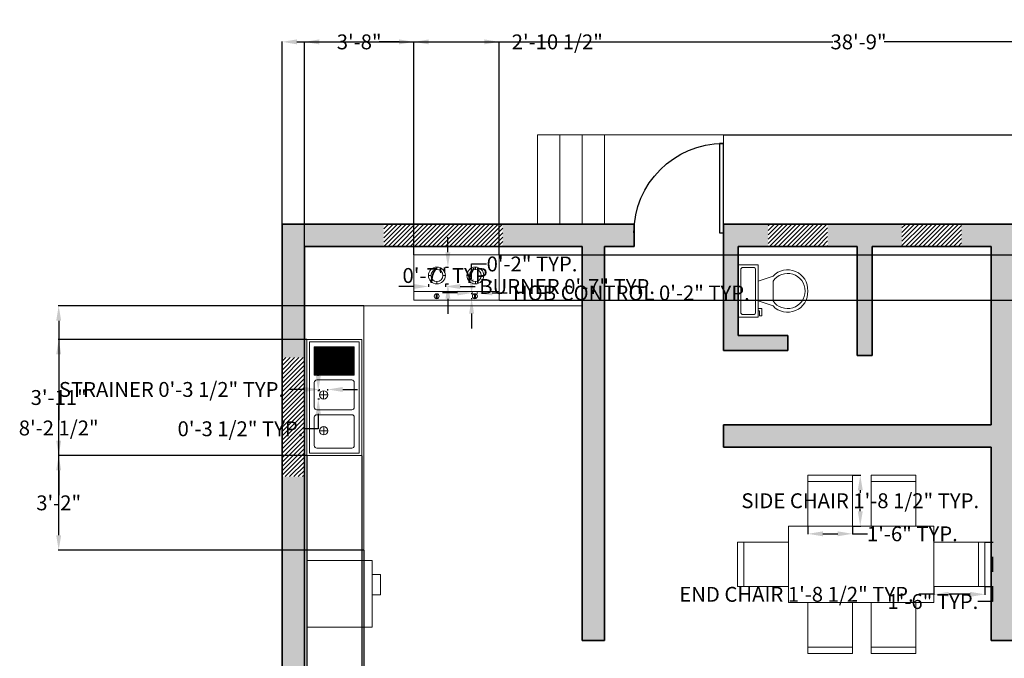
# Model space of a CAD drawing. Units: inches. Extents: x 1966 to 4198, y 2607 to 3884.
# Tile 6 of 8: x 2775 to 3172, y 3625 to 3883. Entities that reach past the tile are written whole.
import ezdxf

# ---------------------------------------------------------------- set-up
doc = ezdxf.new("R2010")
doc.units = ezdxf.units.IN
doc.header["$MEASUREMENT"] = 0
for name, color, linetype, lineweight in [('A-EQPM', 163, 'Continuous', 18), ('A-FIXT-PATT', 163, 'Continuous', 13), ('A-FLOR-CASE', 163, 'Continuous', 18), ('A-FLOR-FIXT', 163, 'Continuous', 18), ('A-FLOR-STRS', 7, 'Continuous', 18), ('A-GLAZ-PATT', 14, 'Continuous', 13), ('A-WALL', 7, 'Continuous', 35), ('A-WALL-PATT', 252, 'Continuous', 13), ('dimension', 90, 'Continuous', 18), ('door', 17, 'Continuous', 25), ('furniture', 163, 'Continuous', 18)]:
    doc.layers.add(name, color=color, linetype=linetype, lineweight=lineweight)
doc.styles.get("Standard").update_dxf_attribs({"font": 'arial.ttf'})
doc.dimstyles.get("Standard").update_dxf_attribs({"dimtxt": 6, "dimasz": 6, "dimexe": 0.18, "dimexo": 0.0625, "dimgap": 0.09, "dimtad": 0, "dimtih": 1, "dimtoh": 1, "dimdec": 1, "dimzin": 0, "dimdsep": 46, "dimlunit": 3, "dimtxsty": 'Standard', "dimcen": 0.09, "dimadec": 0, "dimazin": 0, "dimtfac": 1, "dimtdec": 1, "dimtofl": 0, "dimtmove": 0, "dimatfit": 3, "dimfxl": 1, "dimtolj": 1, "dimtzin": 0, "dimarcsym": 0})

# ---------------------------------------------------------------- blocks, each defined once
blk = doc.blocks.new('*U2')
for p, q in [((0, 0), (0, -6)), ((40, 0), (40, -6))]:
    blk.add_line(p, q)
blk.add_lwpolyline([(0, 0), (0, 40), (1.75, 40), (1.75, 0)], close=True)
blk.add_arc((0, 0), 40, 0, 90)
blk = doc.blocks.new('*U14')
for p, q in [((9.5, -6), (9.5, -2)), ((-10, -8.5), (-8, -8.5)), ((-10, -9.5), (-10, -8.5)), ((-7, -9.5), (-10, -9.5)), ((-8, -8.5), (-8, -8)), ((-7, -8), (-7, -9.5)), ((-4, -8), (-6, -14)), ((4, -8), (6, -14)), ((4, -14), (-4, -14))]:
    blk.add_line(p, q)
blk.add_lwpolyline([(10.5, -8), (10.5, 0), (-10.5, 0), (-10.5, -8)], close=True)
for points in [[(-9.5, -2), (-9.5, -6)], [(8.5, -1), (-8.5, -1)], [(-8.5, -7), (8.5, -7)]]:
    blk.add_lwpolyline(points)
for centre, radius, start, end in [((-8.625, -1.875), 0.8839, 81.8699, 188.1301), ((8.625, -1.875), 0.8839, 351.8699, 98.1301), ((-8.625, -6.125), 0.8839, 171.869898, 278.1301), ((8.625, -6.125), 0.8839, 261.8699, 8.1301), ((-0.4772, -19.9188), 8.0953, 133.01722, 273.38), ((0.0374, -19.8731), 7.127, 124.50543, 269.7), ((-0.0373, -19.8731), 7.127, 270.3, 55.4946), ((0.4773, -19.9188), 8.0953, 266.62, 46.9828)]:
    blk.add_arc(centre, radius, start, end)
blk = doc.blocks.new('REAR-ENTRY-STEPS')
for p, q in [((0, 36), (0, 0)), ((0, 36), (27, 36)), ((9, 36), (9, 0)), ((18, 36), (18, 0)), ((75, 36), (27, 36)), ((27, 36), (27, 0)), ((75, 0), (75, 36))]:
    blk.add_line(p, q)
blk = doc.blocks.new('DINING-CHAIR-SIDE')
for points in [[(0, 18), (18, 18), (18, 20.52), (0, 20.52)], [(0, 0), (18, 0), (18, 18), (0, 18)]]:
    blk.add_lwpolyline(points, close=True)
blk = doc.blocks.new('DINING-CHAIR-END')
for points in [[(2.61, 18), (0, 18), (0, 0), (2.61, 0)], [(2.61, 0), (20.61, 0), (20.61, 18), (2.61, 18)]]:
    blk.add_lwpolyline(points, close=True)
blk = doc.blocks.new('COOKTOP-BURNER')
for p, q in [((3.41, 6.82), (3.41, 5.82)), ((0, 3.41), (1, 3.41)), ((3.41, 1), (3.41, 0)), ((5.82, 3.41), (6.82, 3.41))]:
    blk.add_line(p, q)
for radius in [3.41, 2.41]:
    blk.add_circle((3.41, 3.41), radius)
blk = doc.blocks.new('SINK-STRAINER')
for p, q in [((0, 1.68), (3.35, 1.68)), ((1.68, 0), (1.68, 3.35))]:
    blk.add_line(p, q)
blk.add_circle((1.68, 1.68), 1.68)
blk = doc.blocks.new('HOB-CONTROL')
for p, q in [((0.81, 0.02), (0.81, 2)), ((1.21, 0.02), (1.21, 2))]:
    blk.add_line(p, q)
blk.add_circle((1.01, 1.01), 1.01)
blk = doc.blocks.new('*D47')
at = {"layer": 'Defpoints', "color": 0, "transparency": 16777216}
for p in [(3110.55, 3699.16), (3113.63, 3699.16), (3110.55, 3678.63)]:
    blk.add_point(p, dxfattribs=at)
at = {"layer": 'dimension', "color": 0, "lineweight": -2, "transparency": 16777216}
for p, q in [((3110.61, 3699.16), (3113.81, 3699.16)), ((3113.63, 3693.16), (3113.63, 3692.09)), ((3113.63, 3684.63), (3113.63, 3685.7)), ((3110.61, 3678.63), (3113.81, 3678.63))]:
    blk.add_line(p, q, dxfattribs=at)
at = {"layer": 'dimension', "color": 0, "transparency": 16777216}
for points in [[(3112.63, 3693.16), (3114.63, 3693.16), (3113.63, 3699.16)], [(3112.63, 3684.63), (3114.63, 3684.63), (3113.63, 3678.63)]]:
    blk.add_solid(points, dxfattribs=at)
at = {"layer": 'dimension', "color": 0, "transparency": 16777216, "insert": (3113.63, 3688.9), "char_height": 6, "attachment_point": 5}
blk.add_mtext('\\A1;SIDE CHAIR 1\'-8 1/2" TYP.', dxfattribs=at)
blk = doc.blocks.new('*D48')
at = {"layer": 'Defpoints', "color": 0, "transparency": 16777216}
for p in [(3092.55, 3678.63), (3110.55, 3678.63), (3110.55, 3675.56)]:
    blk.add_point(p, dxfattribs=at)
at = {"layer": 'dimension', "color": 0, "lineweight": -2, "transparency": 16777216}
for p, q in [((3092.55, 3678.57), (3092.55, 3675.38)), ((3110.55, 3678.57), (3110.55, 3675.38)), ((3098.55, 3675.56), (3104.55, 3675.56)), ((3110.55, 3675.56), (3116.55, 3675.56))]:
    blk.add_line(p, q, dxfattribs=at)
at = {"layer": 'dimension', "color": 0, "transparency": 16777216}
for points in [[(3098.55, 3676.56), (3098.55, 3674.56), (3092.55, 3675.56)], [(3104.55, 3676.56), (3104.55, 3674.56), (3110.55, 3675.56)]]:
    blk.add_solid(points, dxfattribs=at)
at = {"layer": 'dimension', "color": 0, "transparency": 16777216, "insert": (3134.65, 3675.56), "char_height": 6, "attachment_point": 5}
blk.add_mtext('\\A1;1\'-6" TYP.', dxfattribs=at)
blk = doc.blocks.new('*D65')
at = {"layer": 'Defpoints', "color": 0, "transparency": 16777216}
for p in [(3143.32, 3654.24), (3163.93, 3654.24), (3143.32, 3651.15)]:
    blk.add_point(p, dxfattribs=at)
at = {"layer": 'dimension', "color": 0, "lineweight": -2, "transparency": 16777216}
for p, q in [((3143.32, 3654.18), (3143.32, 3650.97)), ((3163.93, 3654.18), (3163.93, 3650.97)), ((3143.32, 3651.15), (3137.32, 3651.15)), ((3157.93, 3651.15), (3149.32, 3651.15))]:
    blk.add_line(p, q, dxfattribs=at)
at = {"layer": 'dimension', "color": 0, "transparency": 16777216}
for points in [[(3149.32, 3652.15), (3149.32, 3650.15), (3143.32, 3651.15)], [(3157.93, 3652.15), (3157.93, 3650.15), (3163.93, 3651.15)]]:
    blk.add_solid(points, dxfattribs=at)
at = {"layer": 'dimension', "color": 0, "transparency": 16777216, "insert": (3087.9, 3651.15), "char_height": 6, "attachment_point": 5}
blk.add_mtext('\\A1;END CHAIR 1\'-8 1/2" TYP.', dxfattribs=at)
blk = doc.blocks.new('*D66')
at = {"layer": 'Defpoints', "color": 0, "transparency": 16777216}
for p in [(3163.93, 3672.24), (3163.93, 3654.24), (3167.02, 3654.24)]:
    blk.add_point(p, dxfattribs=at)
at = {"layer": 'dimension', "color": 0, "lineweight": -2, "transparency": 16777216}
for p, q in [((3163.99, 3672.24), (3167.2, 3672.24)), ((3167.02, 3666.24), (3167.02, 3660.24)), ((3163.99, 3654.24), (3167.2, 3654.24)), ((3167.02, 3654.24), (3167.02, 3648.24)), ((3167.02, 3648.24), (3161.02, 3648.24))]:
    blk.add_line(p, q, dxfattribs=at)
at = {"layer": 'dimension', "color": 0, "transparency": 16777216}
for points in [[(3166.02, 3666.24), (3168.02, 3666.24), (3167.02, 3672.24)], [(3166.02, 3660.24), (3168.02, 3660.24), (3167.02, 3654.24)]]:
    blk.add_solid(points, dxfattribs=at)
at = {"layer": 'dimension', "color": 0, "transparency": 16777216, "insert": (3142.92, 3648.24), "char_height": 6, "attachment_point": 5}
blk.add_mtext('\\A1;1\'-6" TYP.', dxfattribs=at)
blk = doc.blocks.new('*D67')
at = {"layer": 'Defpoints', "color": 0, "transparency": 16777216}
for p in [(2939.47, 3776.35), (2946.29, 3776.35), (2946.29, 3775.33)]:
    blk.add_point(p, dxfattribs=at)
at = {"layer": 'dimension', "color": 0, "lineweight": -2, "transparency": 16777216}
for p, q in [((2933.47, 3775.33), (2927.47, 3775.33)), ((2939.47, 3776.29), (2939.47, 3775.15)), ((2946.29, 3776.29), (2946.29, 3775.15)), ((2952.29, 3775.33), (2958.29, 3775.33))]:
    blk.add_line(p, q, dxfattribs=at)
at = {"layer": 'dimension', "color": 0, "transparency": 16777216}
for points in [[(2933.47, 3776.33), (2933.47, 3774.33), (2939.47, 3775.33)], [(2952.29, 3776.33), (2952.29, 3774.33), (2946.29, 3775.33)]]:
    blk.add_solid(points, dxfattribs=at)
at = {"layer": 'dimension', "color": 0, "transparency": 16777216, "insert": (2995.39, 3775.33), "char_height": 6, "attachment_point": 5}
blk.add_mtext('\\A1;BURNER 0\'-7" TYP.', dxfattribs=at)
blk = doc.blocks.new('*D68')
at = {"layer": 'Defpoints', "color": 0, "transparency": 16777216}
for p in [(2946.29, 3783.17), (2947.31, 3783.17), (2946.29, 3776.35)]:
    blk.add_point(p, dxfattribs=at)
at = {"layer": 'dimension', "color": 0, "lineweight": -2, "transparency": 16777216}
for p, q in [((2947.31, 3789.17), (2947.31, 3795.17)), ((2946.35, 3783.17), (2947.49, 3783.17)), ((2946.35, 3776.35), (2947.49, 3776.35)), ((2947.31, 3770.35), (2947.31, 3764.35))]:
    blk.add_line(p, q, dxfattribs=at)
at = {"layer": 'dimension', "color": 0, "transparency": 16777216}
for points in [[(2946.31, 3789.17), (2948.31, 3789.17), (2947.31, 3783.17)], [(2946.31, 3770.35), (2948.31, 3770.35), (2947.31, 3776.35)]]:
    blk.add_solid(points, dxfattribs=at)
at = {"layer": 'dimension', "color": 0, "transparency": 16777216, "insert": (2947.31, 3779.76), "char_height": 6, "attachment_point": 5}
blk.add_mtext('\\A1;0\'-7" TYP.', dxfattribs=at)
blk = doc.blocks.new('*D69')
at = {"layer": 'Defpoints', "color": 0, "transparency": 16777216}
for p in [(2895.52, 3733.79), (2895.52, 3733.29), (2898.88, 3733.29)]:
    blk.add_point(p, dxfattribs=at)
at = {"layer": 'dimension', "color": 0, "lineweight": -2, "transparency": 16777216}
for p, q in [((2889.52, 3733.79), (2883.52, 3733.79)), ((2895.52, 3733.35), (2895.52, 3733.97)), ((2898.88, 3733.35), (2898.88, 3733.97)), ((2904.88, 3733.79), (2910.88, 3733.79))]:
    blk.add_line(p, q, dxfattribs=at)
at = {"layer": 'dimension', "color": 0, "transparency": 16777216}
for points in [[(2889.52, 3734.79), (2889.52, 3732.79), (2895.52, 3733.79)], [(2904.88, 3734.79), (2904.88, 3732.79), (2898.88, 3733.79)]]:
    blk.add_solid(points, dxfattribs=at)
at = {"layer": 'dimension', "color": 0, "transparency": 16777216, "insert": (2835.82, 3733.79), "char_height": 6, "attachment_point": 5}
blk.add_mtext('\\A1;STRAINER 0\'-3 1/2" TYP.', dxfattribs=at)
blk = doc.blocks.new('*D70')
at = {"layer": 'Defpoints', "color": 0, "transparency": 16777216}
for p in [(2895.52, 3733.29), (2895.02, 3729.93), (2895.52, 3729.93)]:
    blk.add_point(p, dxfattribs=at)
at = {"layer": 'dimension', "color": 0, "lineweight": -2, "transparency": 16777216}
for p, q in [((2895.02, 3739.29), (2895.02, 3745.29)), ((2895.46, 3733.29), (2894.84, 3733.29)), ((2895.46, 3729.93), (2894.84, 3729.93)), ((2895.02, 3723.93), (2895.02, 3717.93)), ((2895.02, 3717.93), (2889.02, 3717.93))]:
    blk.add_line(p, q, dxfattribs=at)
at = {"layer": 'dimension', "color": 0, "transparency": 16777216}
for points in [[(2894.02, 3739.29), (2896.02, 3739.29), (2895.02, 3733.29)], [(2894.02, 3723.93), (2896.02, 3723.93), (2895.02, 3729.93)]]:
    blk.add_solid(points, dxfattribs=at)
at = {"layer": 'dimension', "color": 0, "transparency": 16777216, "insert": (2863.65, 3717.93), "char_height": 6, "attachment_point": 5}
blk.add_mtext('\\A1;0\'-3 1/2" TYP.', dxfattribs=at)
blk = doc.blocks.new('*D75')
at = {"layer": 'Defpoints', "color": 0, "transparency": 16777216}
for p in [(2957.17, 3772.41), (2959.19, 3772.72), (2959.19, 3772.41)]:
    blk.add_point(p, dxfattribs=at)
at = {"layer": 'dimension', "color": 0, "lineweight": -2, "transparency": 16777216}
for p, q in [((2957.17, 3772.48), (2957.17, 3772.9)), ((2959.19, 3772.48), (2959.19, 3772.9)), ((2951.17, 3772.72), (2945.17, 3772.72)), ((2965.19, 3772.72), (2971.19, 3772.72))]:
    blk.add_line(p, q, dxfattribs=at)
at = {"layer": 'dimension', "color": 0, "transparency": 16777216}
for points in [[(2951.17, 3773.72), (2951.17, 3771.72), (2957.17, 3772.72)], [(2965.19, 3773.72), (2965.19, 3771.72), (2959.19, 3772.72)]]:
    blk.add_solid(points, dxfattribs=at)
at = {"layer": 'dimension', "color": 0, "transparency": 16777216, "insert": (3021.31, 3772.72), "char_height": 6, "attachment_point": 5}
blk.add_mtext('\\A1;HOB CONTROL 0\'-2" TYP.', dxfattribs=at)
blk = doc.blocks.new('*D76')
at = {"layer": 'Defpoints', "color": 0, "transparency": 16777216}
for p in [(2956.87, 3772.41), (2957.17, 3772.41), (2957.17, 3770.39)]:
    blk.add_point(p, dxfattribs=at)
at = {"layer": 'dimension', "color": 0, "lineweight": -2, "transparency": 16777216}
for p, q in [((2956.87, 3778.41), (2956.87, 3784.41)), ((2956.87, 3784.41), (2962.87, 3784.41)), ((2957.11, 3772.41), (2956.69, 3772.41)), ((2957.11, 3770.39), (2956.69, 3770.39)), ((2956.87, 3764.39), (2956.87, 3758.39))]:
    blk.add_line(p, q, dxfattribs=at)
at = {"layer": 'dimension', "color": 0, "transparency": 16777216}
for points in [[(2955.87, 3778.41), (2957.87, 3778.41), (2956.87, 3772.41)], [(2955.87, 3764.39), (2957.87, 3764.39), (2956.87, 3770.39)]]:
    blk.add_solid(points, dxfattribs=at)
at = {"layer": 'dimension', "color": 0, "transparency": 16777216, "insert": (2981.24, 3784.41), "char_height": 6, "attachment_point": 5}
blk.add_mtext('\\A1;0\'-2" TYP.', dxfattribs=at)
blk = doc.blocks.new('*D87')
at = {"layer": 'Defpoints', "color": 0, "transparency": 16777216}
for p in [(3345.44, 3874), (2880.44, 3800.5), (3345.44, 3800.5)]:
    blk.add_point(p, dxfattribs=at)
at = {"layer": 'dimension', "color": 0, "lineweight": -2, "transparency": 16777216}
for p, q in [((2880.44, 3800.57), (2880.44, 3874.18)), ((2886.44, 3874), (3102.55, 3874)), ((3339.44, 3874), (3123.33, 3874)), ((3345.44, 3800.57), (3345.44, 3874.18))]:
    blk.add_line(p, q, dxfattribs=at)
at = {"layer": 'dimension', "color": 0, "transparency": 16777216}
for points in [[(2886.44, 3875), (2886.44, 3873), (2880.44, 3874)], [(3339.44, 3875), (3339.44, 3873), (3345.44, 3874)]]:
    blk.add_solid(points, dxfattribs=at)
at = {"layer": 'dimension', "color": 0, "transparency": 16777216, "insert": (3112.94, 3874), "char_height": 6, "attachment_point": 5}
blk.add_mtext('\\A1;38\'-9"', dxfattribs=at)
blk = doc.blocks.new('*D88')
at = {"layer": 'Defpoints', "color": 0, "transparency": 16777216}
for p in [(3058.44, 3836.5), (3345.44, 3203.44), (3438.28, 3203.44)]:
    blk.add_point(p, dxfattribs=at)
at = {"layer": 'dimension', "color": 0, "lineweight": -2, "transparency": 16777216}
for p, q in [((3058.5, 3836.5), (3438.46, 3836.5)), ((3438.28, 3830.5), (3438.28, 3523.13)), ((3438.28, 3209.44), (3438.28, 3516.82)), ((3345.5, 3203.44), (3438.46, 3203.44))]:
    blk.add_line(p, q, dxfattribs=at)
at = {"layer": 'dimension', "color": 0, "transparency": 16777216}
for points in [[(3437.28, 3830.5), (3439.28, 3830.5), (3438.28, 3836.5)], [(3437.28, 3209.44), (3439.28, 3209.44), (3438.28, 3203.44)]]:
    blk.add_solid(points, dxfattribs=at)
at = {"layer": 'dimension', "color": 0, "transparency": 16777216, "insert": (3438.28, 3519.97), "char_height": 6, "attachment_point": 5}
blk.add_mtext('\\A1;52\'-9"', dxfattribs=at)
blk = doc.blocks.new('*D90')
at = {"layer": 'Defpoints', "color": 0, "transparency": 16777216}
for p in [(2889.440566, 3668.990639), (2913.440566, 3668.990639), (2913.440566, 3160.931053)]:
    blk.add_point(p, dxfattribs=at)
at = {"layer": 'dimension', "color": 0, "lineweight": -2, "transparency": 16777216}
for p, q in [((2889.440566, 3668.928139), (2889.440566, 3160.751053)), ((2913.440566, 3668.928139), (2913.440566, 3160.751053)), ((2883.440566, 3160.931053), (2877.440566, 3160.931053)), ((2919.440566, 3160.931053), (2925.440566, 3160.931053))]:
    blk.add_line(p, q, dxfattribs=at)
at = {"layer": 'dimension', "color": 0, "transparency": 16777216}
for points in [[(2883.440566, 3161.931053), (2883.440566, 3159.931053), (2889.440566, 3160.931053)], [(2919.440566, 3161.931053), (2919.440566, 3159.931053), (2913.440566, 3160.931053)]]:
    blk.add_solid(points, dxfattribs=at)
at = {"layer": 'dimension', "color": 0, "transparency": 16777216, "insert": (2901.440566, 3160.931053), "char_height": 6, "attachment_point": 5}
blk.add_mtext('\\A1;2\'-0"', dxfattribs=at)
blk = doc.blocks.new('*D91')
at = {"layer": 'Defpoints', "color": 0, "transparency": 16777216}
for p in [(2790.33, 3767.5), (2913.44, 3767.5), (2913.44, 3668.99)]:
    blk.add_point(p, dxfattribs=at)
at = {"layer": 'dimension', "color": 0, "lineweight": -2, "transparency": 16777216}
for p, q in [((2913.38, 3767.5), (2790.15, 3767.5)), ((2790.33, 3761.5), (2790.33, 3721.44)), ((2790.33, 3674.99), (2790.33, 3715.05)), ((2913.38, 3668.99), (2790.15, 3668.99))]:
    blk.add_line(p, q, dxfattribs=at)
at = {"layer": 'dimension', "color": 0, "transparency": 16777216}
for points in [[(2789.33, 3761.5), (2791.33, 3761.5), (2790.33, 3767.5)], [(2789.33, 3674.99), (2791.33, 3674.99), (2790.33, 3668.99)]]:
    blk.add_solid(points, dxfattribs=at)
at = {"layer": 'dimension', "color": 0, "transparency": 16777216, "insert": (2790.33, 3718.25), "char_height": 6, "attachment_point": 5}
blk.add_mtext('\\A1;8\'-2 1/2"', dxfattribs=at)
blk = doc.blocks.new('*D94')
at = {"layer": 'Defpoints', "color": 0, "transparency": 16777216}
for p in [(2967.99, 3874), (2933.61, 3788.06), (2967.99, 3788.06)]:
    blk.add_point(p, dxfattribs=at)
at = {"layer": 'dimension', "color": 0, "lineweight": -2, "transparency": 16777216}
for p, q in [((2933.61, 3788.12), (2933.61, 3874.18)), ((2939.61, 3874), (2961.99, 3874)), ((2967.99, 3788.12), (2967.99, 3874.18)), ((2967.99, 3874), (2973.99, 3874))]:
    blk.add_line(p, q, dxfattribs=at)
at = {"layer": 'dimension', "color": 0, "transparency": 16777216}
for points in [[(2939.61, 3875), (2939.61, 3873), (2933.61, 3874)], [(2961.99, 3875), (2961.99, 3873), (2967.99, 3874)]]:
    blk.add_solid(points, dxfattribs=at)
at = {"layer": 'dimension', "color": 0, "transparency": 16777216, "insert": (2991.43, 3874), "char_height": 6, "attachment_point": 5}
blk.add_mtext('\\A1;2\'-10 1/2"', dxfattribs=at)
blk = doc.blocks.new('*D95')
at = {"layer": 'Defpoints', "color": 0, "transparency": 16777216}
for p in [(2933.61, 3874), (2889.44, 3791.5), (2933.61, 3788.06)]:
    blk.add_point(p, dxfattribs=at)
at = {"layer": 'dimension', "color": 0, "lineweight": -2, "transparency": 16777216}
for p, q in [((2889.44, 3791.57), (2889.44, 3874.18)), ((2895.44, 3874), (2903.46, 3874)), ((2927.61, 3874), (2919.59, 3874)), ((2933.61, 3788.12), (2933.61, 3874.18))]:
    blk.add_line(p, q, dxfattribs=at)
at = {"layer": 'dimension', "color": 0, "transparency": 16777216}
for points in [[(2895.44, 3875), (2895.44, 3873), (2889.44, 3874)], [(2927.61, 3875), (2927.61, 3873), (2933.61, 3874)]]:
    blk.add_solid(points, dxfattribs=at)
at = {"layer": 'dimension', "color": 0, "transparency": 16777216, "insert": (2911.52, 3874), "char_height": 6, "attachment_point": 5}
blk.add_mtext('\\A1;3\'-8"', dxfattribs=at)
blk = doc.blocks.new('*D96')
at = {"layer": 'Defpoints', "color": 0, "transparency": 16777216}
for p in [(2967.99, 3788.06), (3438.28, 3788.06), (2967.99, 3769.8)]:
    blk.add_point(p, dxfattribs=at)
at = {"layer": 'dimension', "color": 0, "lineweight": -2, "transparency": 16777216}
for p, q in [((3438.28, 3788.06), (3438.28, 3794.06)), ((3438.28, 3794.06), (3444.28, 3794.06)), ((2968.06, 3788.06), (3438.46, 3788.06)), ((3438.28, 3775.8), (3438.28, 3782.06)), ((2968.06, 3769.8), (3438.46, 3769.8))]:
    blk.add_line(p, q, dxfattribs=at)
at = {"layer": 'dimension', "color": 0, "transparency": 16777216}
for points in [[(3437.28, 3782.06), (3439.28, 3782.06), (3438.28, 3788.06)], [(3437.28, 3775.8), (3439.28, 3775.8), (3438.28, 3769.8)]]:
    blk.add_solid(points, dxfattribs=at)
at = {"layer": 'dimension', "color": 0, "transparency": 16777216, "insert": (3459.06, 3794.06), "char_height": 6, "attachment_point": 5}
blk.add_mtext('\\A1;1\'-6 1/2"', dxfattribs=at)
blk = doc.blocks.new('*D97')
at = {"layer": 'Defpoints', "color": 0, "transparency": 16777216}
for p in [(2890.43, 3707.11), (2912.55, 3707.11), (2912.55, 3160.93)]:
    blk.add_point(p, dxfattribs=at)
at = {"layer": 'dimension', "color": 0, "lineweight": -2, "transparency": 16777216}
for p, q in [((2890.43, 3707.05), (2890.43, 3160.75)), ((2912.55, 3707.05), (2912.55, 3160.75)), ((2884.43, 3160.93), (2878.43, 3160.93)), ((2918.55, 3160.93), (2924.55, 3160.93))]:
    blk.add_line(p, q, dxfattribs=at)
at = {"layer": 'dimension', "color": 0, "transparency": 16777216}
for points in [[(2884.43, 3161.93), (2884.43, 3159.93), (2890.43, 3160.93)], [(2918.55, 3161.93), (2918.55, 3159.93), (2912.55, 3160.93)]]:
    blk.add_solid(points, dxfattribs=at)
at = {"layer": 'dimension', "color": 0, "transparency": 16777216, "insert": (2901.49, 3160.93), "char_height": 6, "attachment_point": 5}
blk.add_mtext('\\A1;1\'-10"', dxfattribs=at)
blk = doc.blocks.new('*D98')
at = {"layer": 'Defpoints', "color": 0, "transparency": 16777216}
for p in [(2790.33, 3753.97), (2890.43, 3753.97), (2890.43, 3707.11)]:
    blk.add_point(p, dxfattribs=at)
at = {"layer": 'dimension', "color": 0, "lineweight": -2, "transparency": 16777216}
for p, q in [((2890.36, 3753.97), (2790.15, 3753.97)), ((2790.33, 3747.97), (2790.33, 3733.7)), ((2790.33, 3713.11), (2790.33, 3727.38)), ((2890.36, 3707.11), (2790.15, 3707.11))]:
    blk.add_line(p, q, dxfattribs=at)
at = {"layer": 'dimension', "color": 0, "transparency": 16777216}
for points in [[(2789.33, 3747.97), (2791.33, 3747.97), (2790.33, 3753.97)], [(2789.33, 3713.11), (2791.33, 3713.11), (2790.33, 3707.11)]]:
    blk.add_solid(points, dxfattribs=at)
at = {"layer": 'dimension', "color": 0, "transparency": 16777216, "insert": (2790.33, 3730.54), "char_height": 6, "attachment_point": 5}
blk.add_mtext('\\A1;3\'-11"', dxfattribs=at)
blk = doc.blocks.new('*D99')
at = {"layer": 'Defpoints', "color": 0, "transparency": 16777216}
for p in [(2890.43, 3707.11), (2790.33, 3668.99), (2889.44, 3668.99)]:
    blk.add_point(p, dxfattribs=at)
at = {"layer": 'dimension', "color": 0, "lineweight": -2, "transparency": 16777216}
for p, q in [((2890.36, 3707.11), (2790.15, 3707.11)), ((2790.33, 3701.11), (2790.33, 3691.21)), ((2790.33, 3674.99), (2790.33, 3684.9)), ((2889.38, 3668.99), (2790.15, 3668.99))]:
    blk.add_line(p, q, dxfattribs=at)
at = {"layer": 'dimension', "color": 0, "transparency": 16777216}
for points in [[(2789.33, 3701.11), (2791.33, 3701.11), (2790.33, 3707.11)], [(2789.33, 3674.99), (2791.33, 3674.99), (2790.33, 3668.99)]]:
    blk.add_solid(points, dxfattribs=at)
at = {"layer": 'dimension', "color": 0, "transparency": 16777216, "insert": (2790.33, 3688.05), "char_height": 6, "attachment_point": 5}
blk.add_mtext('\\A1;3\'-2"', dxfattribs=at)

msp = doc.modelspace()

# ---------------------------------------------------------------- hatches: boundary and pattern name
at = {"layer": 'A-FIXT-PATT'}
h = msp.add_hatch(dxfattribs=at)
h.set_pattern_fill('ANSI31', color=256, scale=2.4, angle=315, style=0)
h.paths.add_polyline_path([(2893.43, 3739.61), (2909.55, 3739.61), (2909.55, 3750.97), (2893.43, 3750.97)])
at = {"layer": 'A-GLAZ-PATT'}
h = msp.add_hatch(dxfattribs=at)
h.set_pattern_fill('ANSI31', color=256, scale=10)
h.set_pattern_definition([(45, (819.9656, 0), (-0.88388348, 0.88388348), [])])
h.paths.add_polyline_path([(2884.94, 3746.62), (2880.44, 3746.62), (2880.44, 3698.62), (2884.94, 3698.62)])
h.paths.add_polyline_path([(2889.44, 3746.62), (2884.94, 3746.62), (2884.94, 3698.62), (2889.44, 3698.62)])
h.paths.add_polyline_path([(2969.44, 3800.5), (2921.44, 3800.5), (2921.44, 3796), (2969.44, 3796)])
h.paths.add_polyline_path([(2969.44, 3796), (2921.44, 3796), (2921.44, 3791.5), (2969.44, 3791.5)])
h.paths.add_polyline_path([(3100.44, 3800.5), (3076.44, 3800.5), (3076.44, 3796), (3100.44, 3796)])
h.paths.add_polyline_path([(3100.44, 3796), (3076.44, 3796), (3076.44, 3791.5), (3100.44, 3791.5)])
h.paths.add_polyline_path([(3154.44, 3800.5), (3130.44, 3800.5), (3130.44, 3796), (3154.44, 3796)])
h.paths.add_polyline_path([(3154.44, 3796), (3130.44, 3796), (3130.44, 3791.5), (3154.44, 3791.5)])
h.paths.add_polyline_path([(3279.94, 3800.5), (3231.94, 3800.5), (3231.94, 3796), (3279.94, 3796)])
h.paths.add_polyline_path([(3279.94, 3796), (3231.94, 3796), (3231.94, 3791.5), (3279.94, 3791.5)])
h.paths.add_polyline_path([(3345.44, 3740.5), (3340.94, 3740.5), (3340.94, 3692.5), (3345.44, 3692.5)])
h.paths.add_polyline_path([(3340.94, 3740.5), (3336.44, 3740.5), (3336.44, 3692.5), (3340.94, 3692.5)])
h.paths.add_polyline_path([(3340.94, 3626.5), (3336.44, 3626.5), (3336.44, 3602.5), (3340.94, 3602.5)])
h.paths.add_polyline_path([(3345.44, 3626.5), (3340.94, 3626.5), (3340.94, 3602.5), (3345.44, 3602.5)])
h.paths.add_polyline_path([(3345.44, 3538), (3340.94, 3538), (3340.94, 3490), (3345.44, 3490)])
h.paths.add_polyline_path([(3340.94, 3538), (3336.44, 3538), (3336.44, 3490), (3340.94, 3490)])
h.paths.add_polyline_path([(3280.44, 3436), (3232.44, 3436), (3232.44, 3431.5), (3280.44, 3431.5)])
h.paths.add_polyline_path([(3280.44, 3440.5), (3232.44, 3440.5), (3232.44, 3436), (3280.44, 3436)])
at = {"layer": 'A-WALL-PATT'}
h = msp.add_hatch(color=256, dxfattribs=at)
h.dxf.hatch_style = 1
h.paths.add_polyline_path([(3010.44, 3599.5), (2889.44, 3599.5), (2889.44, 3698.62), (2880.44, 3698.62), (2880.44, 3590.5), (2880.44, 3539.5), (2889.44, 3539.5), (2889.44, 3590.5), (3010.44, 3590.5)])
h.paths.add_polyline_path([(2889.44, 3491.5), (2880.44, 3491.5), (2880.44, 3431.5), (2924.93, 3431.5), (2924.93, 3440.5), (2889.44, 3440.5)])
h.paths.add_polyline_path([(3008.43, 3440.5), (2972.93, 3440.5), (2972.93, 3431.5), (3008.43, 3431.5)])
h.paths.add_polyline_path([(2995.02, 3431.5), (2991.02, 3431.5), (2991.02, 3345.5), (3014.67, 3345.5), (3014.67, 3349.5), (2995.02, 3349.5)])
h.paths.add_polyline_path([(3232.44, 3440.5), (3176.44, 3440.5), (3176.44, 3587.5), (3183.92, 3587.5), (3183.92, 3591.41), (3183.92, 3596.5), (3167.44, 3596.5), (3167.44, 3440.5), (3092.44, 3440.5), (3092.44, 3590.5), (3083.44, 3590.5), (3083.44, 3440.5), (3056.43, 3440.5), (3056.43, 3438.68), (3056.43, 3431.5), (3092.44, 3431.5), (3232.44, 3431.5)])
h.paths.add_polyline_path([(3176.44, 3431.5), (3172.44, 3431.5), (3172.44, 3349.5), (3074.67, 3349.5), (3074.67, 3345.5), (3176.44, 3345.5)])
h.paths.add_polyline_path([(3345.44, 3490), (3336.44, 3490), (3336.44, 3440.5), (3280.44, 3440.5), (3280.44, 3431.5), (3345.44, 3431.5)])
h.paths.add_polyline_path([(3345.44, 3599.5), (3345.44, 3602.5), (3336.44, 3602.5), (3336.44, 3596.5), (3296.55, 3596.5), (3296.55, 3587.5), (3336.44, 3587.5), (3336.44, 3538), (3345.44, 3538)])
h.paths.add_polyline_path([(3264.44, 3632.5), (3336.44, 3632.5), (3336.44, 3626.5), (3345.44, 3626.5), (3345.44, 3692.5), (3336.44, 3692.5), (3336.44, 3641.5), (3219.92, 3641.5), (3219.92, 3632.5), (3258.44, 3632.5), (3258.44, 3596.5), (3219.95, 3596.5), (3219.95, 3591.41, -0.010779), (3219.92, 3589.86), (3219.92, 3587.5), (3268.55, 3587.5), (3268.55, 3591.7), (3268.55, 3596.5), (3264.44, 3596.5)])
h.paths.add_polyline_path([(3175.44, 3791.5), (3231.94, 3791.5), (3231.94, 3800.5), (3175.44, 3800.5), (3154.44, 3800.5), (3154.44, 3791.5), (3166.44, 3791.5), (3166.44, 3719.5), (3118.44, 3719.5), (3112.44, 3719.5), (3058.44, 3719.5), (3058.44, 3710.5), (3166.44, 3710.5), (3166.44, 3632.5), (3183.92, 3632.5), (3183.92, 3637.87), (3183.92, 3641.5), (3175.44, 3641.5)])
h.paths.add_polyline_path([(3345.44, 3800.5), (3279.94, 3800.5), (3279.94, 3791.5), (3336.44, 3791.5), (3336.44, 3740.5), (3345.44, 3740.5)])
h.paths.add_polyline_path([(3130.44, 3800.5), (3100.44, 3800.5), (3100.44, 3791.5), (3112.44, 3791.5), (3112.44, 3755.5), (3112.44, 3751.71), (3112.44, 3747.5), (3118.44, 3747.5), (3118.44, 3791.5), (3130.44, 3791.5)], flags=17)
h.paths.add_polyline_path([(3076.44, 3800.5), (3058.44, 3800.5), (3058.44, 3796.92), (3058.44, 3791.5), (3058.44, 3749.5), (3084.38, 3749.5), (3084.38, 3751.71, -0.016709), (3084.44, 3753.59), (3084.44, 3755.5), (3064.44, 3755.5), (3064.44, 3791.5), (3076.44, 3791.5)], flags=17)
h.paths.add_polyline_path([(3022.36, 3796.92, -0.017138), (3022.44, 3799.39), (3022.44, 3800.5), (3010.44, 3800.5), (2969.44, 3800.5), (2969.44, 3791.5), (3001.44, 3791.5), (3001.44, 3632.5), (3010.44, 3632.5), (3010.44, 3791.5), (3022.36, 3791.5)])
h.paths.add_polyline_path([(2921.44, 3800.5), (2880.44, 3800.5), (2880.44, 3746.62), (2889.44, 3746.62), (2889.44, 3791.5), (2921.44, 3791.5)])

# ---------------------------------------------------------------- linework, layer by layer
at = {"layer": 'A-EQPM'}
msp.add_line((2933.61, 3773.27), (2967.99, 3773.27), dxfattribs=at)
for points in [[(2933.61, 3788.06), (2967.99, 3788.06), (2967.99, 3769.8), (2933.61, 3769.8)], [(2890.61, 3664.86), (2916.71, 3664.86), (2916.71, 3637.84), (2890.61, 3637.84)], [(2916.71, 3659.1), (2920.19, 3659.1), (2920.19, 3650.88), (2916.71, 3650.88)]]:
    msp.add_lwpolyline(points, close=True, dxfattribs=at)
at = {"layer": 'A-FLOR-CASE'}
for p, q in [((3001.44, 3767.5), (2913.44, 3767.5)), ((2913.44, 3767.5), (2913.44, 3668.99)), ((2913.44, 3668.99), (2889.44, 3668.99))]:
    msp.add_line(p, q, dxfattribs=at)
at = {"layer": 'A-FLOR-FIXT'}
msp.add_line((2893.43, 3739.61), (2909.55, 3739.61), dxfattribs=at)
for points in [[(2890.43, 3753.97), (2912.55, 3753.97), (2912.55, 3707.11), (2890.43, 3707.11)], [(2891.43, 3752.97), (2911.55, 3752.97), (2911.55, 3708.11), (2891.43, 3708.11)]]:
    msp.add_lwpolyline(points, close=True, dxfattribs=at)
msp.add_lwpolyline([(2893.43, 3739.61), (2893.43, 3750.97), (2909.55, 3750.97), (2909.55, 3739.61)], dxfattribs=at)
for points in [[(2893.43, 3726.61), (2893.43, 3736.61, -0.414214), (2894.43, 3737.61), (2908.55, 3737.61, -0.414214), (2909.55, 3736.61), (2909.55, 3726.61, -0.414214), (2908.55, 3725.61), (2894.43, 3725.61, -0.414214)], [(2909.55, 3722.61), (2909.55, 3711.11, -0.414214), (2908.55, 3710.11), (2894.43, 3710.11, -0.414214), (2893.43, 3711.11), (2893.43, 3722.61, -0.414214), (2894.43, 3723.61), (2908.55, 3723.61, -0.414214)]]:
    msp.add_lwpolyline(points, format="xyb", close=True, dxfattribs=at)
at = {"layer": 'A-WALL'}
for p, q in [((3022.44, 3800.5), (2880.44, 3800.5)), ((2880.44, 3800.5), (2880.44, 3590.5)), ((3022.44, 3791.5), (3022.44, 3800.5)), ((3175.44, 3800.5), (3058.44, 3800.5)), ((3058.44, 3791.5), (3058.44, 3800.5)), ((3001.44, 3791.5), (2889.44, 3791.5)), ((2889.44, 3791.5), (2889.44, 3599.5)), ((3001.44, 3632.5), (3001.44, 3791.5)), ((3010.44, 3632.5), (3010.44, 3791.5)), ((3022.44, 3791.5), (3010.44, 3791.5)), ((3058.44, 3749.5), (3058.44, 3791.5)), ((3064.44, 3755.5), (3064.44, 3791.5)), ((3112.44, 3791.5), (3064.44, 3791.5)), ((3112.44, 3755.5), (3112.44, 3791.5)), ((3118.44, 3747.5), (3118.44, 3791.5)), ((3166.44, 3791.5), (3118.44, 3791.5)), ((3166.44, 3719.5), (3166.44, 3791.5)), ((3084.44, 3755.5), (3064.44, 3755.5)), ((3084.44, 3749.5), (3084.44, 3755.5)), ((3112.44, 3749.5), (3112.44, 3755.5)), ((3084.44, 3749.5), (3058.44, 3749.5)), ((3112.44, 3747.5), (3112.44, 3749.5)), ((3112.44, 3747.5), (3118.44, 3747.5)), ((3058.44, 3710.5), (3058.44, 3719.5)), ((3112.44, 3719.5), (3058.44, 3719.5)), ((3112.44, 3719.5), (3118.44, 3719.5)), ((3166.44, 3719.5), (3118.44, 3719.5)), ((3166.44, 3710.5), (3058.44, 3710.5)), ((3166.44, 3632.5), (3166.44, 3710.5)), ((3001.44, 3632.5), (3010.44, 3632.5)), ((3166.44, 3632.5), (3183.92, 3632.5))]:
    msp.add_line(p, q, dxfattribs=at)
at = {"layer": 'furniture'}
msp.add_lwpolyline([(3084.68, 3678.63), (3143.32, 3678.63), (3143.32, 3647.85), (3084.68, 3647.85)], close=True, dxfattribs=at)

# ---------------------------------------------------------------- block references
at = {"layer": 'A-EQPM'}
for name, p in [('COOKTOP-BURNER', (2939.47, 3776.35)), ('HOB-CONTROL', (2941.78, 3770.39)), ('HOB-CONTROL', (2957.17, 3770.39))]:
    msp.add_blockref(name, p, dxfattribs=at)
at = {"layer": 'A-EQPM', "rotation": 90.00000000000765}
msp.add_blockref('COOKTOP-BURNER', (2961.79, 3776.35), dxfattribs=at)
at = {"layer": 'A-FLOR-FIXT'}
for name, p, rotation in [('*U14', (3064.44, 3773.5), 89.99999999999999), ('SINK-STRAINER', (2898.88, 3733.29), 180)]:
    msp.add_blockref(name, p, dxfattribs=dict(at, rotation=rotation))
msp.add_blockref('SINK-STRAINER', (2895.53, 3715.43), dxfattribs=at)
at = {"layer": 'A-FLOR-STRS'}
msp.add_blockref('REAR-ENTRY-STEPS', (2983.44, 3800.5), dxfattribs=at)
at = {"layer": 'door', "xscale": -0.902118520811191, "yscale": 0.902118520811191, "zscale": 0.902118520811191}
msp.add_blockref('*U2', (3058.44, 3796.92), dxfattribs=at)
at = {"layer": 'furniture'}
for name, p in [('DINING-CHAIR-SIDE', (3092.55, 3678.63)), ('DINING-CHAIR-SIDE', (3118.07, 3678.63)), ('DINING-CHAIR-END', (3064.07, 3654.24))]:
    msp.add_blockref(name, p, dxfattribs=at)
at = {"layer": 'furniture', "rotation": 180}
msp.add_blockref('DINING-CHAIR-END', (3163.93, 3672.24), dxfattribs=at)
at = {"layer": 'furniture', "extrusion": (0, 0, -1), "zscale": -1, "rotation": 180}
for p in [(-3092.55, 3647.85), (-3118.07, 3647.85)]:
    msp.add_blockref('DINING-CHAIR-SIDE', p, dxfattribs=at)

# ---------------------------------------------------------------- dimensions: what is measured, and where the dimension line sits
at = {"layer": 'dimension'}
for base, p1, p2, picture, middle in [((2967.99, 3874), (2933.61, 3788.06), (2967.99, 3788.06), '*D94', (2991.43, 3874)), ((3345.44, 3874), (2880.44, 3800.5), (3345.44, 3800.5), '*D87', (3112.94, 3874)), ((2933.61, 3874), (2889.44, 3791.5), (2933.61, 3788.06), '*D95', (2911.52, 3874)), ((2912.55, 3160.93), (2890.43, 3707.11), (2912.55, 3707.11), '*D97', (2901.49, 3160.93)), ((2913.44, 3160.93), (2889.44, 3668.99), (2913.44, 3668.99), '*D90', (2901.44, 3160.93))]:
    dim = msp.add_linear_dim(base=base, p1=p1, p2=p2, dimstyle='Standard', override={"dimdec": 1, "dimlfac": 1, "dimrnd": 0, "dimzin": 1, "dimdsep": 46, "dimlunit": 4, "dimfrac": 2}, dxfattribs=at)
    dim.commit()
    dim.dimension.update_dxf_attribs({"geometry": picture, "text_midpoint": middle})
for base, p1, p2, picture, middle in [((3438.28, 3203.44), (3058.44, 3836.5), (3345.44, 3203.44), '*D88', (3438.28, 3519.97)), ((3438.28, 3788.06), (2967.99, 3769.8), (2967.99, 3788.06), '*D96', (3459.06, 3794.06)), ((2790.33, 3767.5), (2913.44, 3668.99), (2913.44, 3767.5), '*D91', (2790.33, 3718.25)), ((2790.33, 3753.97), (2890.43, 3707.11), (2890.43, 3753.97), '*D98', (2790.33, 3730.54)), ((2790.33, 3668.99), (2890.43, 3707.11), (2889.44, 3668.99), '*D99', (2790.33, 3688.05))]:
    dim = msp.add_linear_dim(base=base, p1=p1, p2=p2, angle=90, dimstyle='Standard', override={"dimdec": 1, "dimlfac": 1, "dimrnd": 0, "dimzin": 1, "dimdsep": 46, "dimlunit": 4, "dimfrac": 2}, dxfattribs=at)
    dim.commit()
    dim.dimension.update_dxf_attribs({"geometry": picture, "text_midpoint": middle})
for base, p1, p2, angle, text, picture, middle in [((2947.31, 3783.17), (2946.29, 3776.35), (2946.29, 3783.17), 90, '<> TYP.', '*D68', (2947.31, 3779.76)), ((2956.87, 3772.41), (2957.17, 3770.39), (2957.17, 3772.41), 90, '<> TYP.', '*D76', (2981.24, 3784.41)), ((2895.52, 3733.79), (2898.88, 3733.29), (2895.52, 3733.29), 180, 'STRAINER <> TYP.', '*D69', (2835.82, 3733.79)), ((2895.02, 3729.93), (2895.52, 3733.29), (2895.52, 3729.93), 270, '<> TYP.', '*D70', (2863.65, 3717.93)), ((3113.63, 3699.16), (3110.55, 3678.63), (3110.55, 3699.16), 90, 'SIDE CHAIR <> TYP.', '*D47', (3113.63, 3688.9)), ((3143.32, 3651.15), (3163.93, 3654.24), (3143.32, 3654.24), 180, 'END CHAIR <> TYP.', '*D65', (3087.9, 3651.15)), ((3167.02, 3654.24), (3163.93, 3672.24), (3163.93, 3654.24), 270, '<> TYP.', '*D66', (3142.92, 3648.24))]:
    dim = msp.add_linear_dim(base=base, p1=p1, p2=p2, angle=angle, text=text, dimstyle='Standard', override={"dimdec": 1, "dimlfac": 1, "dimrnd": 0, "dimzin": 1, "dimdsep": 46, "dimlunit": 4, "dimfrac": 2}, dxfattribs=at)
    dim.commit()
    dim.dimension.update_dxf_attribs({"geometry": picture, "text_midpoint": middle})
for base, p1, p2, text, picture, middle in [((2946.29, 3775.33), (2939.47, 3776.35), (2946.29, 3776.35), 'BURNER <> TYP.', '*D67', (2995.39, 3775.33)), ((2959.19, 3772.72), (2957.17, 3772.41), (2959.19, 3772.41), 'HOB CONTROL <> TYP.', '*D75', (3021.31, 3772.72)), ((3110.55, 3675.56), (3092.55, 3678.63), (3110.55, 3678.63), '<> TYP.', '*D48', (3134.65, 3675.56))]:
    dim = msp.add_linear_dim(base=base, p1=p1, p2=p2, text=text, dimstyle='Standard', override={"dimdec": 1, "dimlfac": 1, "dimrnd": 0, "dimzin": 1, "dimdsep": 46, "dimlunit": 4, "dimfrac": 2}, dxfattribs=at)
    dim.commit()
    dim.dimension.update_dxf_attribs({"geometry": picture, "text_midpoint": middle})

doc.saveas('drawing.dxf')
